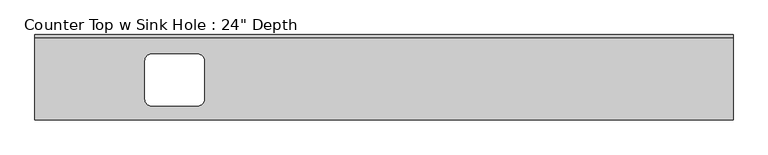
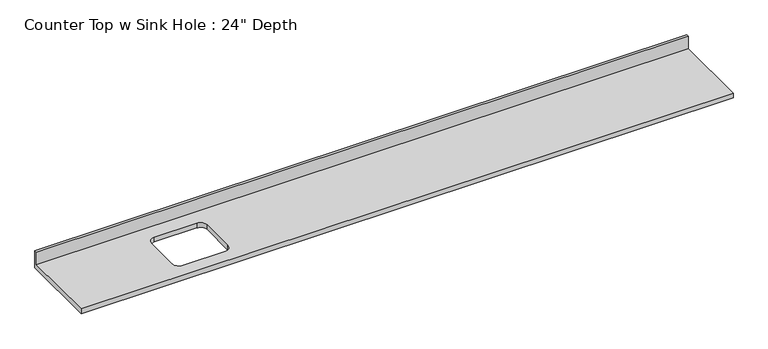
"""IFC4 building model written with IfcOpenShell, lengths in millimetres: furniture geometry."""

from ifc_helpers import new_model, si_unit, frame, origin, place, context, project, spatial, polyline, circle_curve, source, transform, mapped, element, save
from ifc_brep_helpers import plane_surface, revolved_surface, advanced_brep


def furniture_d6024f60(model_context):
    return source(origin(), model_context, "Body", "AdvancedBrep", [
        advanced_brep(
        [(-1200.4622951, -622.3, 914.4), (3879.5377049, -622.3, 914.4), (3879.5377049, -19.05, 914.4), (-1200.4622951, -19.05, 914.4), (-349.5622951, -139.7, 914.4), (-19.3622951, -139.7, 914.4), (31.4377049, -190.5, 914.4), (31.4377049, -469.9, 914.4), (-19.3622951, -520.7, 914.4), (-349.5622951, -520.7, 914.4), (-400.3622951, -469.9, 914.4), (-400.3622951, -190.5, 914.4), (3879.5377049, 0.0, 876.3), (3879.5377049, -622.3, 876.3), (-1200.4622951, -622.3, 876.3), (-1200.4622951, 0.0, 876.3), (-19.3622951, -139.7, 876.3), (-349.5622951, -139.7, 876.3), (-400.3622951, -190.5, 876.3), (-400.3622951, -469.9, 876.3), (-349.5622951, -520.7, 876.3), (-19.3622951, -520.7, 876.3), (31.4377049, -469.9, 876.3), (31.4377049, -190.5, 876.3), (-1200.4622951, 0.0, 1016.0), (3879.5377049, 0.0, 1016.0), (-1200.4622951, -19.05, 1016.0), (3879.5377049, -19.05, 1016.0)],
        [
            (0, 1),
            (1, 2),
            (2, 3),
            (3, 0),
            (4, 5),
            (5, 6, circle_curve(frame((-19.3622951, -190.5, 914.4), z_axis=(0.0, 0.0, -1.0), x_axis=(1.0, 0.0, 0.0)), 50.8)),
            (6, 7),
            (7, 8, circle_curve(frame((-19.3622951, -469.9, 914.4), z_axis=(0.0, 0.0, -1.0), x_axis=(1.0, 0.0, 0.0)), 50.8)),
            (8, 9),
            (9, 10, circle_curve(frame((-349.5622951, -469.9, 914.4), z_axis=(0.0, 0.0, -1.0), x_axis=(1.0, 0.0, 0.0)), 50.8)),
            (10, 11),
            (11, 4, circle_curve(frame((-349.5622951, -190.5, 914.4), z_axis=(0.0, 0.0, -1.0), x_axis=(1.0, 0.0, 0.0)), 50.8)),
            (12, 13),
            (13, 14),
            (14, 15),
            (15, 12),
            (16, 17),
            (17, 18, circle_curve(frame((-349.5622951, -190.5, 876.3), z_axis=(0.0, 0.0, 1.0), x_axis=(1.0, 0.0, 0.0)), 50.8)),
            (18, 19),
            (19, 20, circle_curve(frame((-349.5622951, -469.9, 876.3), z_axis=(0.0, 0.0, 1.0), x_axis=(1.0, 0.0, 0.0)), 50.8)),
            (20, 21),
            (21, 22, circle_curve(frame((-19.3622951, -469.9, 876.3), z_axis=(0.0, 0.0, 1.0), x_axis=(1.0, 0.0, 0.0)), 50.8)),
            (22, 23),
            (23, 16, circle_curve(frame((-19.3622951, -190.5, 876.3), z_axis=(0.0, 0.0, 1.0), x_axis=(1.0, 0.0, 0.0)), 50.8)),
            (15, 24),
            (24, 25),
            (25, 12),
            (14, 0),
            (3, 26),
            (26, 24),
            (13, 1),
            (25, 27),
            (27, 2),
            (4, 17),
            (16, 5),
            (11, 18),
            (10, 19),
            (9, 20),
            (8, 21),
            (7, 22),
            (6, 23),
            (26, 27),
        ],
        [
            plane_surface(frame((-1200.4622951, 0.0, 914.4), z_axis=(0.0, 0.0, 1.0), x_axis=(-1.0, 0.0, 0.0))),
            plane_surface(frame((-1200.4622951, 0.0, 876.3), z_axis=(0.0, 0.0, -1.0), x_axis=(1.0, 0.0, 0.0))),
            plane_surface(frame((3879.5377049, 0.0, 914.4), z_axis=(0.0, 1.0, 0.0), x_axis=(0.0, 0.0, -1.0))),
            plane_surface(frame((-1200.4622951, 0.0, 914.4), z_axis=(-1.0, 0.0, 0.0), x_axis=(0.0, 0.0, -1.0))),
            plane_surface(frame((-1200.4622951, -622.3, 914.4), z_axis=(0.0, -1.0, 0.0), x_axis=(0.0, 0.0, -1.0))),
            plane_surface(frame((3879.5377049, -622.3, 914.4), z_axis=(1.0, 0.0, 0.0), x_axis=(0.0, 0.0, -1.0))),
            plane_surface(frame((-19.3622951, -139.7, 914.4), z_axis=(0.0, -1.0, 0.0), x_axis=(0.0, 0.0, -1.0))),
            revolved_surface(polyline([(-298.76229509999996, -190.5, 914.4), (-298.76229509999996, -190.5, 876.3)]), (-349.5622951, -190.5, 876.3), (0.0, 0.0, 1.0)),
            plane_surface(frame((-400.3622951, -190.5, 914.4), z_axis=(1.0, 0.0, 0.0), x_axis=(0.0, 0.0, -1.0))),
            revolved_surface(polyline([(-298.76229509999996, -469.9, 914.4), (-298.76229509999996, -469.9, 876.3)]), (-349.5622951, -469.9, 876.3), (0.0, 0.0, 1.0)),
            plane_surface(frame((-349.5622951, -520.7, 914.4), z_axis=(0.0, 1.0, 0.0), x_axis=(0.0, 0.0, -1.0))),
            revolved_surface(polyline([(31.437704899999996, -469.9, 914.4), (31.437704899999996, -469.9, 876.3)]), (-19.3622951, -469.9, 876.3), (0.0, 0.0, 1.0)),
            plane_surface(frame((31.4377049, -469.9, 914.4), z_axis=(-1.0, 0.0, 0.0), x_axis=(0.0, 0.0, -1.0))),
            revolved_surface(polyline([(31.437704899999996, -190.5, 914.4), (31.437704899999996, -190.5, 876.3)]), (-19.3622951, -190.5, 876.3), (0.0, 0.0, 1.0)),
            plane_surface(frame((-1200.4622951, 0.0, 1016.0), z_axis=(0.0, 0.0, 1.0), x_axis=(0.0, -1.0, 0.0))),
            plane_surface(frame((-1200.4622951, -19.05, 1016.0), z_axis=(0.0, -1.0, 0.0), x_axis=(0.0, 0.0, -1.0))),
        ],
        [
            (0, [[1, 2, 3, 4], [5, 6, 7, 8, 9, 10, 11, 12]]),
            (1, [[13, 14, 15, 16], [17, 18, 19, 20, 21, 22, 23, 24]]),
            (2, [[-16, 25, 26, 27]]),
            (3, [[-15, 28, -4, 29, 30, -25]]),
            (4, [[-1, -28, -14, 31]]),
            (5, [[-13, -27, 32, 33, -2, -31]]),
            (6, [[34, -17, 35, -5]]),
            (7, [[-34, -12, 36, -18]]),
            (8, [[-36, -11, 37, -19]]),
            (9, [[-37, -10, 38, -20]]),
            (10, [[-38, -9, 39, -21]]),
            (11, [[-39, -8, 40, -22]]),
            (12, [[-40, -7, 41, -23]]),
            (13, [[-35, -24, -41, -6]]),
            (14, [[-30, 42, -32, -26]]),
            (15, [[-42, -29, -3, -33]]),
        ],
    ),
    ])


if __name__ == "__main__":
    model = new_model("IFC4")
    model_context = context("Model", 3, world=origin())
    ifc_project = project(units=[si_unit("LENGTHUNIT", "METRE", prefix="MILLI")], contexts=[model_context])
    site = spatial("IfcSite", under=ifc_project)
    building = spatial("IfcBuilding", under=site)
    placement = place(None, origin())
    furniture_shape = furniture_d6024f60(model_context)
    element("IfcFurniture", 1, ObjectType="Counter Top w Sink Hole : 24\" Depth", at=placement, inside=building, context=model_context, shape_type="MappedRepresentation", body=[
        mapped(furniture_shape, transform((0.0, 0.0, 0.0), x_axis=(1.0, 0.0, 0.0), y_axis=(0.0, 1.0, 0.0), z_axis=(0.0, 0.0, 1.0))),
    ])
    save(model, "model.ifc")

# Revit data of these elements
# Type "Counter Top w Sink Hole : 24\" Depth"
#   Assembly Code = "C1030400"
#   Counter Thickness = 0' - 1 1/2"
#   Depth [instance default] = 2' - 1"
#   Height = 3' - 0"
#   Length [instance default] = 8' - 0"
#   Sink Location [instance default] = 2' - 0"
#   Sink Location To Wall [instance default] = 0' - 6"
#   Sink Opening Depth [instance default] = 1' - 3"
#   Sink Opening Width [instance default] = 2' - 3"
#   Counter Top Material = none
#   Default Elevation = 0
# Element 1 (IfcFurniture, "Counter Top w Sink Hole : 24\" Depth")
#   Depth = 2' - 0 1/2"
#   Length = 16' - 8"
#   Sink Location = 3' - 4"
#   Sink Opening Depth = 1' - 2"
#   Sink Opening Width = 1' - 4"
#   Materials on its faces: "Counter Top"
# Materials
#   "Counter Top": class "Wood", colour RGB 226 177 128, transparency 0
